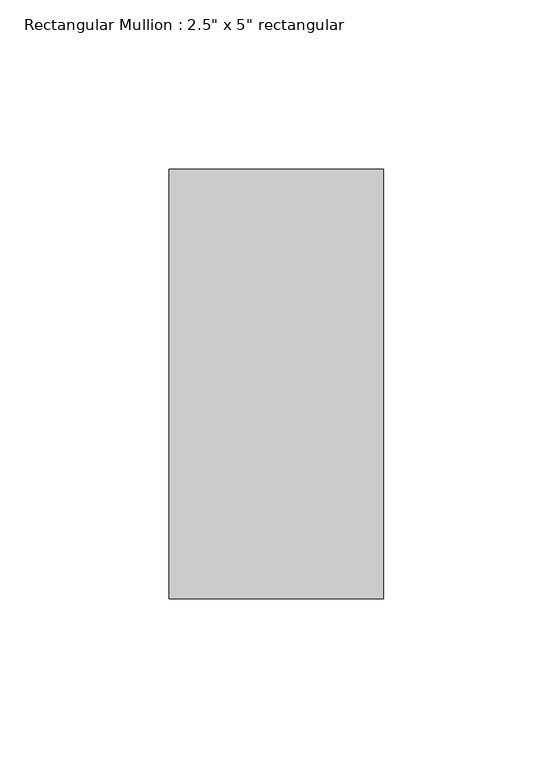
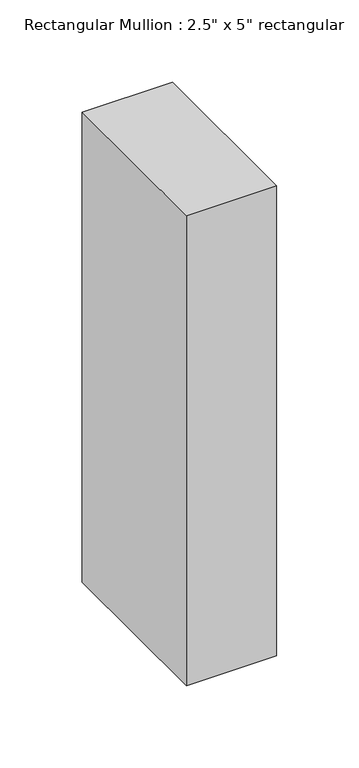
"""IFC4 building model written with IfcOpenShell, lengths in millimetres: member geometry."""

from ifc_helpers import new_model, si_unit, frame, origin, place, context, project, spatial, polyline, outline, extrude, source, transform, mapped, element, save


def member_285f5b4f(model_context):
    return source(origin(), model_context, "Body", "SweptSolid", [
        extrude(outline(polyline([(0.0, 63.5), (0.0, -63.5), (-63.5, -63.5), (-63.5, 63.5), (0.0, 63.5)])), frame((0.0, 0.0, -349.25), z_axis=(0.0, 0.0, 1.0), x_axis=(1.0, 0.0, 0.0)), (0.0, 0.0, 1.0), 349.25),
    ])


if __name__ == "__main__":
    model = new_model("IFC4")
    model_context = context("Model", 3, world=origin())
    ifc_project = project(units=[si_unit("LENGTHUNIT", "METRE", prefix="MILLI")], contexts=[model_context])
    site = spatial("IfcSite", under=ifc_project)
    building = spatial("IfcBuilding", under=site)
    placement = place(None, origin())
    member_shape = member_285f5b4f(model_context)
    element("IfcMember", 1, ObjectType="Rectangular Mullion : 2.5\" x 5\" rectangular", at=placement, inside=building, context=model_context, shape_type="MappedRepresentation", body=[
        mapped(member_shape, transform((0.0, 0.0, 0.0), x_axis=(1.0, 0.0, 0.0), y_axis=(0.0, 1.0, 0.0), z_axis=(0.0, 0.0, 1.0))),
    ])
    save(model, "model.ifc")

# Revit data of these elements
# Type "Rectangular Mullion : 2.5\" x 5\" rectangular"
#   built-in parameter 1007304 = 0.416667 (stored number, unit not read)
#   built-in parameter 1007301 = 0.104167 (stored number, unit not read)
#   built-in parameter 1007300 = 0.104167 (stored number, unit not read)
# Element 1 (IfcMember, "Rectangular Mullion : 2.5\" x 5\" rectangular")
#   Materials on its faces: "Aluminum"
# Materials
#   "Aluminum": class "Metal", colour RGB 247 247 247, transparency 0, Description = "Aluminum 6061", Cost = 0
